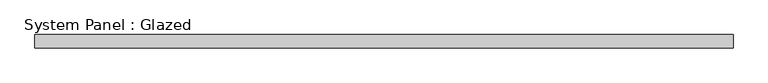
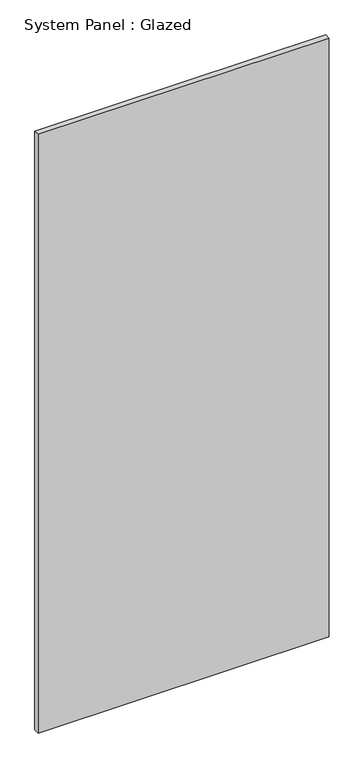
"""IFC4 building model written with IfcOpenShell, lengths in millimetres: plate geometry, System Panel : Glazed."""

from ifc_helpers import new_model, si_unit, origin, origin_with_axes, place, context, project, spatial, polyline, outline, extrude, source, transform, mapped, element, save


def system_panel_glazed_7b556abe(model_context):
    return source(origin(), model_context, "Body", "SweptSolid", [
        extrude(outline(polyline([(671.9413255, 19.05), (-671.9413255, 19.05), (-671.9413255, 44.45), (671.9413255, 44.45), (671.9413255, 19.05)])), origin_with_axes(), (0.0, 0.0, 1.0), 2921.0),
    ])


if __name__ == "__main__":
    model = new_model("IFC4")
    model_context = context("Model", 3, world=origin())
    ifc_project = project(units=[si_unit("LENGTHUNIT", "METRE", prefix="MILLI")], contexts=[model_context])
    site = spatial("IfcSite", under=ifc_project)
    building = spatial("IfcBuilding", under=site)
    placement = place(None, origin())
    system_panel_glazed_shape = system_panel_glazed_7b556abe(model_context)
    element("IfcPlate", 1, ObjectType="System Panel : Glazed", at=placement, inside=building, context=model_context, shape_type="MappedRepresentation", body=[
        mapped(system_panel_glazed_shape, transform((0.0, 0.0, 0.0), x_axis=(1.0, 0.0, 0.0), y_axis=(0.0, 1.0, 0.0), z_axis=(0.0, 0.0, 1.0))),
    ])
    save(model, "model.ifc")

# Revit data of these elements
# Type "System Panel : Glazed"
#   Construction Type Id = "GSP4R"
#   Analytic Construction = "1/8 in Pilkington single glazing"
#   Visual Light Transmittance = 0.9
#   Solar Heat Gain Coefficient = 0.86
#   Heat Transfer Coefficient (U) = 1.18115 BTU/(h·ft²·°F)
# Element 1 (IfcPlate, "System Panel : Glazed")
#   Materials on its faces: "Glass"
# Materials
#   "Glass": class "Glass", colour RGB 0 128 192, transparency 0.75, Description = "Soda Lime Glass", Cost = 0
